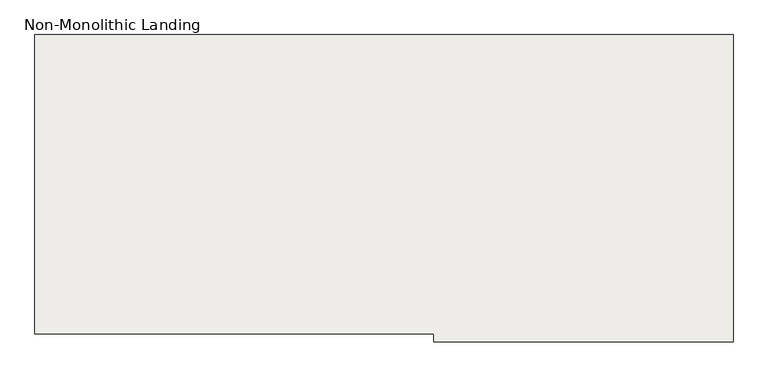
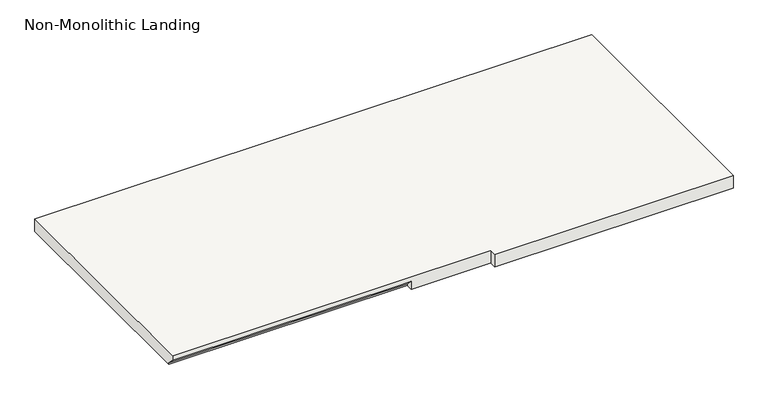
"""IFC4 building model written with IfcOpenShell, lengths in millimetres: slab geometry, Non-Monolithic Landing."""

from ifc_helpers import new_model, si_unit, origin, place, context, project, spatial, faceted_brep, source, transform, mapped, element, save


def non_monolithic_landing_2a8916bf(model_context):
    return source(origin(), model_context, "Body", "Brep", [
        faceted_brep([(-3617.4415084, 23194.7216096, 30464.9005799), (-3617.4415084, 23220.1216096, 30439.5005799), (-2703.0415084, 23220.1216096, 30439.5005799), (-2703.0415084, 23194.7216096, 30464.9005799), (-2398.2415084, 23194.7216096, 30483.9505799), (-2398.2415084, 23169.3216096, 30483.9505799), (-1483.8415084, 23169.3216096, 30483.9505799), (-1483.8415084, 23194.7216096, 30483.9505799), (-1483.8415084, 24109.1216096, 30483.9505799), (-3617.4415084, 24109.1216096, 30483.9505799), (-3617.4415084, 23194.7216096, 30483.9505799), (-2703.0415084, 23220.1216096, 30433.1505799), (-3617.4415084, 23220.1216096, 30433.1505799), (-3617.4415084, 24109.1216096, 30433.1505799), (-1483.8415084, 24109.1216096, 30433.1505799), (-1483.8415084, 23194.7216096, 30433.1505799), (-1483.8415084, 23169.3216096, 30433.1505799), (-2398.2415084, 23169.3216096, 30433.1505799), (-2398.2415084, 23194.7216096, 30433.1505799), (-2703.0415084, 23194.7216096, 30433.1505799)], [[[0, 1, 2, 3]], [[4, 5, 6, 7, 8, 9, 10]], [[11, 12, 13, 14, 15, 16, 17, 18, 19]], [[12, 11, 2, 1]], [[11, 19, 3, 2]], [[4, 10, 0, 3, 19, 18]], [[5, 4, 18, 17]], [[6, 5, 17, 16]], [[7, 6, 16, 15]], [[8, 7, 15, 14]], [[9, 8, 14, 13]], [[10, 9, 13, 12, 1, 0]]]),
    ])


if __name__ == "__main__":
    model = new_model("IFC4")
    model_context = context("Model", 3, world=origin())
    ifc_project = project(units=[si_unit("LENGTHUNIT", "METRE", prefix="MILLI")], contexts=[model_context])
    site = spatial("IfcSite", under=ifc_project)
    building = spatial("IfcBuilding", under=site)
    placement = place(None, origin())
    non_monolithic_landing_shape = non_monolithic_landing_2a8916bf(model_context)
    element("IfcSlab", 1, ObjectType="Non-Monolithic Landing", at=placement, inside=building, context=model_context, shape_type="MappedRepresentation", body=[
        mapped(non_monolithic_landing_shape, transform((0.0, 0.0, 0.0), x_axis=(1.0, 0.0, 0.0), y_axis=(0.0, 1.0, 0.0), z_axis=(0.0, 0.0, 1.0))),
    ])
    save(model, "model.ifc")
